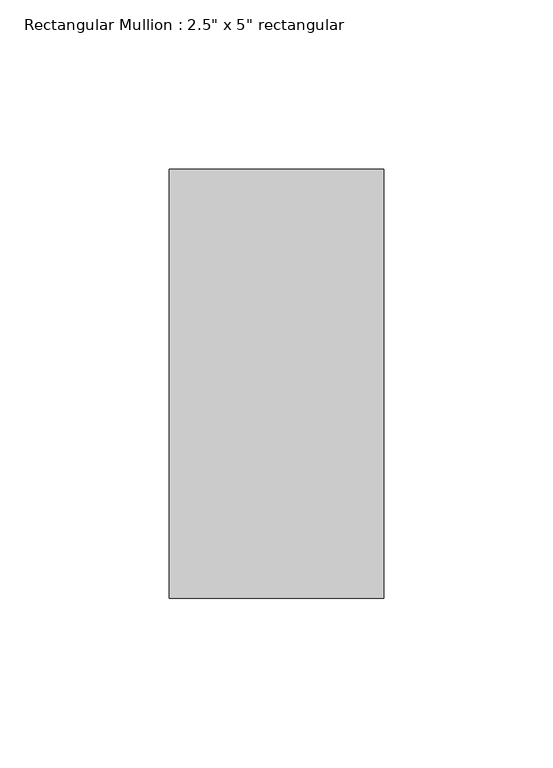
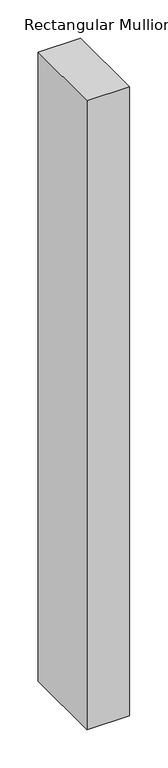
"""IFC4 building model written with IfcOpenShell, lengths in millimetres: member geometry."""

from ifc_helpers import new_model, si_unit, frame, origin, place, context, project, spatial, polyline, outline, extrude, source, transform, mapped, element, save


def member_769db2f1(model_context):
    return source(origin(), model_context, "Body", "SweptSolid", [
        extrude(outline(polyline([(0.0, 63.5), (0.0, -63.5), (-63.5, -63.5), (-63.5, 63.5), (0.0, 63.5)])), frame((0.0, 0.0, -997.961214), z_axis=(0.0, 0.0, 1.0), x_axis=(1.0, 0.0, 0.0)), (0.0, 0.0, 1.0), 997.961214),
    ])


if __name__ == "__main__":
    model = new_model("IFC4")
    model_context = context("Model", 3, world=origin())
    ifc_project = project(units=[si_unit("LENGTHUNIT", "METRE", prefix="MILLI")], contexts=[model_context])
    site = spatial("IfcSite", under=ifc_project)
    building = spatial("IfcBuilding", under=site)
    placement = place(None, origin())
    member_shape = member_769db2f1(model_context)
    element("IfcMember", 1, ObjectType="Rectangular Mullion : 2.5\" x 5\" rectangular", at=placement, inside=building, context=model_context, shape_type="MappedRepresentation", body=[
        mapped(member_shape, transform((0.0, 0.0, 0.0), x_axis=(1.0, 0.0, 0.0), y_axis=(0.0, 1.0, 0.0), z_axis=(0.0, 0.0, 1.0))),
    ])
    save(model, "model.ifc")

# Revit data of these elements
# Type "Rectangular Mullion : 2.5\" x 5\" rectangular"
#   built-in parameter 1007304 = 0.416667 (stored number, unit not read)
#   built-in parameter 1007301 = 0.104167 (stored number, unit not read)
#   built-in parameter 1007300 = 0.104167 (stored number, unit not read)
# Element 1 (IfcMember, "Rectangular Mullion : 2.5\" x 5\" rectangular")
#   Materials on its faces: "Aluminum"
# Materials
#   "Aluminum": class "Metal", colour RGB 247 247 247, transparency 0, Description = "Aluminum 6061", Cost = 0
